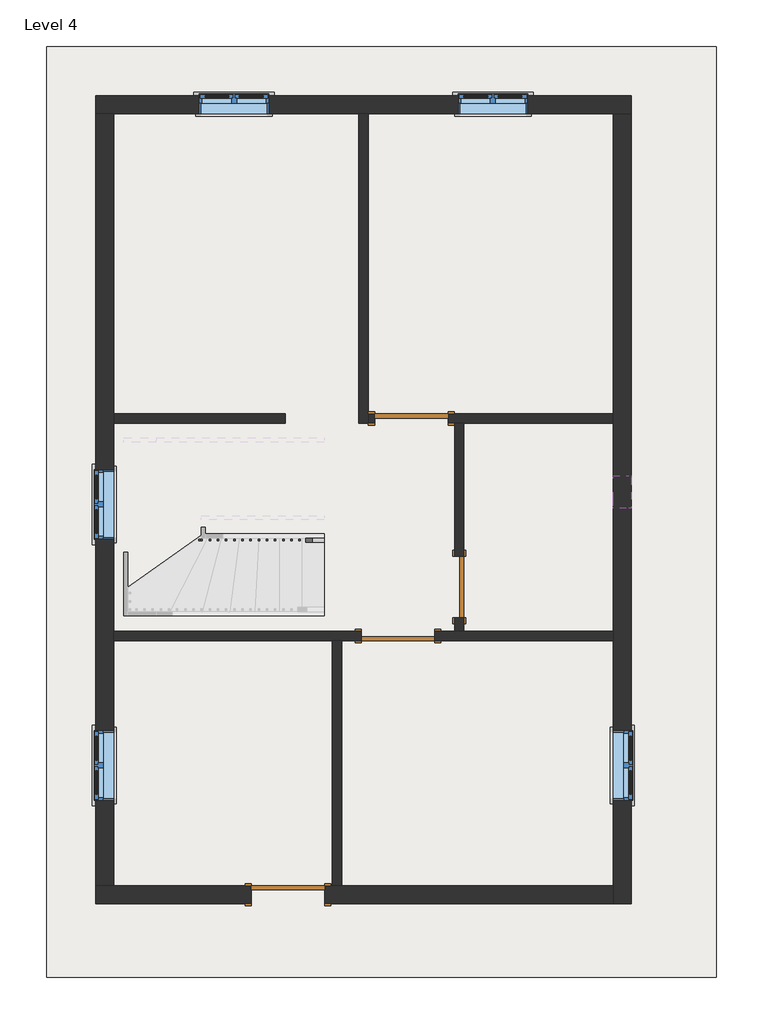
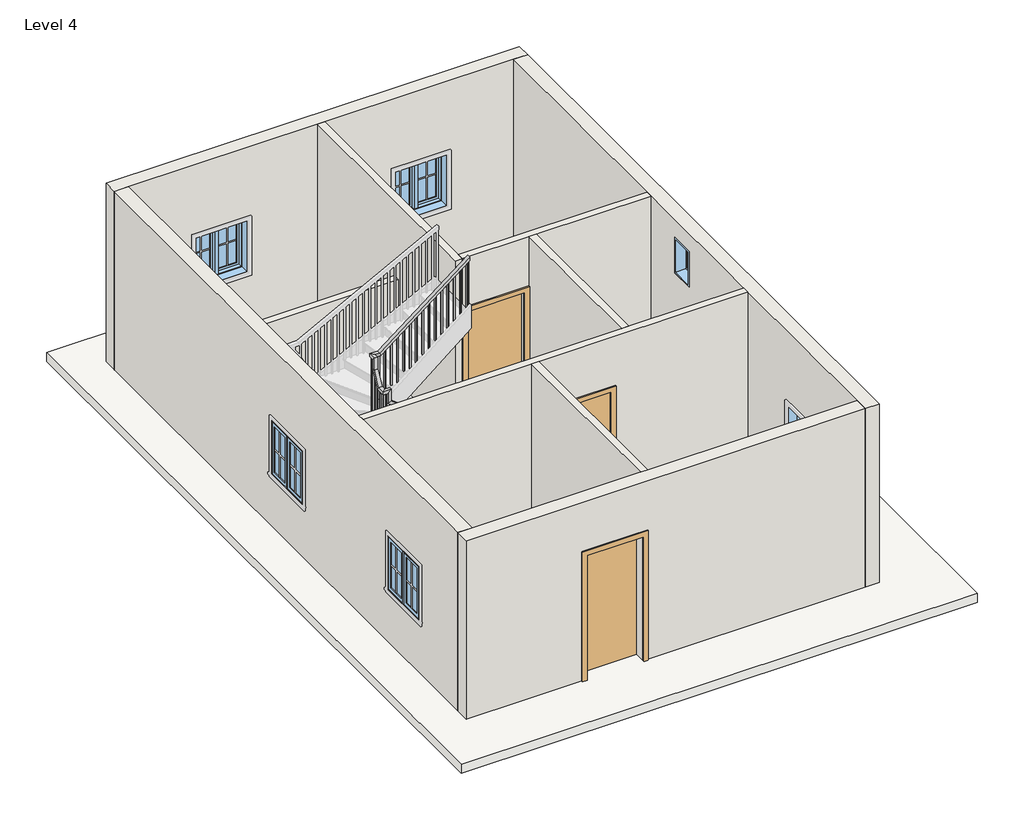
# One storey, part 1 of 2: 10 walls, 6 windows, 4 doors, 1 railing, 1 roof.
"""IFC4 building model written with IfcOpenShell, lengths in millimetres."""

from ifc_helpers import new_model, si_unit, frame, origin, place, context, project, spatial, polyline, outline, extrude, faceted_brep, transform, mapped, element, save
from components import door_d8f5dbb5, door_305aa2a5, door_e5f9f3c4, door_a90ba1ad, window_aa618e30, window_339605e1

model = new_model("IFC4")

# Units and contexts
model_context = context("Model", 3, world=origin())
ifc_project = project(units=[si_unit("LENGTHUNIT", "METRE", prefix="MILLI")], contexts=[model_context])

# Site, building, storey
site = spatial("IfcSite", under=ifc_project)
building = spatial("IfcBuilding", under=site)
storey = spatial("IfcBuildingStorey", under=building, Name="Level 4", Elevation=6400.8)

# Doors
placement = place(None, origin())
door_shape = door_d8f5dbb5(model_context)
element("IfcDoor", 1, ObjectType="Single-Flush : 30\" x 80\"", at=placement, inside=storey, context=model_context, shape_type="MappedRepresentation", body=[
    mapped(door_shape, transform((-82.2715692, -955.3070853, 6400.8), x_axis=(0.0, -1.0, 0.0), y_axis=(1.0, 0.0, 0.0), z_axis=(0.0, 0.0, 1.0))),
])
door_2_shape = door_305aa2a5(model_context)
element("IfcDoor", 2, ObjectType="Single-Flush : 36\" x 84\"", at=placement, inside=storey, context=model_context, shape_type="MappedRepresentation", body=[
    mapped(door_2_shape, transform((-677.5332429, 1140.1929147, 6400.8), x_axis=(-1.0, 0.0, 0.0), y_axis=(0.0, -1.0, 0.0), z_axis=(0.0, 0.0, 1.0))),
])
door_3_shape = door_e5f9f3c4(model_context)
element("IfcDoor", 3, ObjectType="Single-Flush : 36\" x 84\"", at=placement, inside=storey, context=model_context, shape_type="MappedRepresentation", body=[
    mapped(door_3_shape, transform((-842.6332429, -1564.9070853, 6400.8), x_axis=(-1.0, 0.0, 0.0), y_axis=(0.0, -1.0, 0.0), z_axis=(0.0, 0.0, 1.0))),
])
door_4_shape = door_a90ba1ad(model_context)
element("IfcDoor", 4, ObjectType="Single-Flush : 36\" x 84\"", at=placement, inside=storey, context=model_context, shape_type="MappedRepresentation", body=[
    mapped(door_4_shape, transform((-2212.5949167, -4784.3570853, 6400.8), x_axis=(-1.0, 0.0, 0.0), y_axis=(0.0, -1.0, 0.0), z_axis=(0.0, 0.0, 1.0))),
])

# Railing
element("IfcRailing", 5, ObjectType="Handrail - Rectangular", at=placement, inside=storey, context=model_context, shape_type="SolidModel", body=[
    faceted_brep([(-1761.7449167, -396.5070853, 7484.5333333), (-1761.7449167, -396.5070853, 7420.2000346), (-1761.7449167, -345.7070853, 7420.2000346), (-1761.7449167, -345.7070853, 7484.5333333), (-3213.2766085, -396.5070853, 8612.4191036), (-3264.0766085, -396.5070853, 8587.5590024), (-3264.0766085, -345.7070853, 8587.5590024), (-3213.2766085, -345.7070853, 8612.4191036), (-3213.2766085, -396.5070853, 8815.4281882), (-3264.0766085, -396.5070853, 8764.6281882), (-3264.0766085, -345.7070853, 8764.6281882), (-3213.2766085, -345.7070853, 8815.4281882), (-3340.2766085, -396.5070853, 8815.4281882), (-3340.2766085, -396.5070853, 8764.6281882), (-3289.4766085, -345.7070853, 8764.6281882), (-3289.4766085, -345.7070853, 8815.4281882), (-3340.2766085, -269.5070853, 8815.4281882), (-3340.2766085, -240.3857515, 8764.6281882), (-3289.4766085, -240.3857515, 8764.6281882), (-3289.4766085, -269.5070853, 8815.4281882), (-3340.2766085, -142.5070853, 9032.3051451), (-3340.2766085, -91.7070853, 9018.5256424), (-3289.4766085, -91.7070853, 9018.5256424), (-3289.4766085, -142.5070853, 9032.3051451), (-3340.2766085, -142.5070853, 9235.3142297), (-3340.2766085, -91.7070853, 9184.5142297), (-3289.4766085, -91.7070853, 9184.5142297), (-3289.4766085, -142.5070853, 9235.3142297), (-3340.2766085, -15.5070853, 9235.3142297), (-3340.2766085, -15.5070853, 9184.5142297), (-3289.4766085, -66.3070853, 9184.5142297), (-3289.4766085, -66.3070853, 9235.3142297), (-3213.2766085, -15.5070853, 9235.3142297), (-3195.8599406, -15.5070853, 9184.5142297), (-3195.8599406, -66.3070853, 9184.5142297), (-3213.2766085, -66.3070853, 9235.3142297), (-1761.7449167, -15.5070853, 10363.2), (-1761.7449167, -66.3070853, 10363.2), (-1761.7449167, -66.3070853, 10298.8667013), (-1761.7449167, -15.5070853, 10298.8667013)], [[[0, 1, 2, 3]], [[1, 0, 4, 5]], [[2, 1, 5, 6]], [[3, 2, 6, 7]], [[0, 3, 7, 4]], [[5, 4, 8, 9]], [[6, 5, 9, 10]], [[7, 6, 10, 11]], [[4, 7, 11, 8]], [[9, 8, 12, 13]], [[10, 9, 13, 14]], [[11, 10, 14, 15]], [[8, 11, 15, 12]], [[13, 12, 16, 17]], [[14, 13, 17, 18]], [[15, 14, 18, 19]], [[12, 15, 19, 16]], [[17, 16, 20, 21]], [[18, 17, 21, 22]], [[19, 18, 22, 23]], [[16, 19, 23, 20]], [[21, 20, 24, 25]], [[22, 21, 25, 26]], [[23, 22, 26, 27]], [[20, 23, 27, 24]], [[25, 24, 28, 29]], [[26, 25, 29, 30]], [[27, 26, 30, 31]], [[24, 27, 31, 28]], [[29, 28, 32, 33]], [[30, 29, 33, 34]], [[31, 30, 34, 35]], [[28, 31, 35, 32]], [[36, 37, 38, 39]], [[33, 32, 36, 39]], [[34, 33, 39, 38]], [[35, 34, 38, 37]], [[32, 35, 37, 36]]]),
    extrude(outline(polyline([(10283.6316852, -1781.3516085), (10268.8292361, -1800.4016085), (9279.4666667, -1800.4016085), (9279.4666667, -1781.3516085), (10283.6316852, -1781.3516085)])), frame((0.0, -50.4320853, 0.0), z_axis=(0.0, 1.0, 0.0), x_axis=(0.0, 0.0, 1.0)), (0.0, 0.0, 1.0), 19.05),
    extrude(outline(polyline([(10204.6852902, -1882.9516085), (10189.8828411, -1902.0016085), (9279.4666667, -1902.0016085), (9279.4666667, -1882.9516085), (10204.6852902, -1882.9516085)])), frame((0.0, -50.4320853, 0.0), z_axis=(0.0, 1.0, 0.0), x_axis=(0.0, 0.0, 1.0)), (0.0, 0.0, 1.0), 19.05),
    extrude(outline(polyline([(10125.7388952, -1984.5516085), (10110.9364462, -2003.6016085), (9279.4666667, -2003.6016085), (9279.4666667, -1984.5516085), (10125.7388952, -1984.5516085)])), frame((0.0, -50.4320853, 0.0), z_axis=(0.0, 1.0, 0.0), x_axis=(0.0, 0.0, 1.0)), (0.0, 0.0, 1.0), 19.05),
    extrude(outline(polyline([(10046.7925003, -2086.1516085), (10031.9900512, -2105.2016085), (9110.1333333, -2105.2016085), (9110.1333333, -2086.1516085), (10046.7925003, -2086.1516085)])), frame((0.0, -50.4320853, 0.0), z_axis=(0.0, 1.0, 0.0), x_axis=(0.0, 0.0, 1.0)), (0.0, 0.0, 1.0), 19.05),
    extrude(outline(polyline([(9967.8461053, -2187.7516085), (9953.0436562, -2206.8016085), (9110.1333333, -2206.8016085), (9110.1333333, -2187.7516085), (9967.8461053, -2187.7516085)])), frame((0.0, -50.4320853, 0.0), z_axis=(0.0, 1.0, 0.0), x_axis=(0.0, 0.0, 1.0)), (0.0, 0.0, 1.0), 19.05),
    extrude(outline(polyline([(9888.8997103, -2289.3516085), (9874.0972613, -2308.4016085), (9110.1333333, -2308.4016085), (9110.1333333, -2289.3516085), (9888.8997103, -2289.3516085)])), frame((0.0, -50.4320853, 0.0), z_axis=(0.0, 1.0, 0.0), x_axis=(0.0, 0.0, 1.0)), (0.0, 0.0, 1.0), 19.05),
    extrude(outline(polyline([(9809.9533154, -2390.9516085), (9795.1508663, -2410.0016085), (8940.8, -2410.0016085), (8940.8, -2390.9516085), (9809.9533154, -2390.9516085)])), frame((0.0, -50.4320853, 0.0), z_axis=(0.0, 1.0, 0.0), x_axis=(0.0, 0.0, 1.0)), (0.0, 0.0, 1.0), 19.05),
    extrude(outline(polyline([(9731.0069204, -2492.5516085), (9716.2044713, -2511.6016085), (8940.8, -2511.6016085), (8940.8, -2492.5516085), (9731.0069204, -2492.5516085)])), frame((0.0, -50.4320853, 0.0), z_axis=(0.0, 1.0, 0.0), x_axis=(0.0, 0.0, 1.0)), (0.0, 0.0, 1.0), 19.05),
    extrude(outline(polyline([(9652.0605254, -2594.1516085), (9637.2580764, -2613.2016085), (8771.4666667, -2613.2016085), (8771.4666667, -2594.1516085), (9652.0605254, -2594.1516085)])), frame((0.0, -50.4320853, 0.0), z_axis=(0.0, 1.0, 0.0), x_axis=(0.0, 0.0, 1.0)), (0.0, 0.0, 1.0), 19.05),
    extrude(outline(polyline([(9573.1141304, -2695.7516085), (9558.3116814, -2714.8016085), (8771.4666667, -2714.8016085), (8771.4666667, -2695.7516085), (9573.1141304, -2695.7516085)])), frame((0.0, -50.4320853, 0.0), z_axis=(0.0, 1.0, 0.0), x_axis=(0.0, 0.0, 1.0)), (0.0, 0.0, 1.0), 19.05),
    extrude(outline(polyline([(9494.1677355, -2797.3516085), (9479.3652864, -2816.4016085), (8771.4666667, -2816.4016085), (8771.4666667, -2797.3516085), (9494.1677355, -2797.3516085)])), frame((0.0, -50.4320853, 0.0), z_axis=(0.0, 1.0, 0.0), x_axis=(0.0, 0.0, 1.0)), (0.0, 0.0, 1.0), 19.05),
    extrude(outline(polyline([(9415.2213405, -2898.9516085), (9400.4188914, -2918.0016085), (8602.1333333, -2918.0016085), (8602.1333333, -2898.9516085), (9415.2213405, -2898.9516085)])), frame((0.0, -50.4320853, 0.0), z_axis=(0.0, 1.0, 0.0), x_axis=(0.0, 0.0, 1.0)), (0.0, 0.0, 1.0), 19.05),
    extrude(outline(polyline([(9336.2749455, -3000.5516085), (9321.4724965, -3019.6016085), (8602.1333333, -3019.6016085), (8602.1333333, -3000.5516085), (9336.2749455, -3000.5516085)])), frame((0.0, -50.4320853, 0.0), z_axis=(0.0, 1.0, 0.0), x_axis=(0.0, 0.0, 1.0)), (0.0, 0.0, 1.0), 19.05),
    extrude(outline(polyline([(9257.3285506, -3102.1516085), (9242.5261015, -3121.2016085), (8432.8, -3121.2016085), (8432.8, -3102.1516085), (9257.3285506, -3102.1516085)])), frame((0.0, -50.4320853, 0.0), z_axis=(0.0, 1.0, 0.0), x_axis=(0.0, 0.0, 1.0)), (0.0, 0.0, 1.0), 19.05),
    extrude(outline(polyline([(9178.3821556, -3203.7516085), (9163.5797065, -3222.8016085), (8432.8, -3222.8016085), (8432.8, -3203.7516085), (9178.3821556, -3203.7516085)])), frame((0.0, -50.4320853, 0.0), z_axis=(0.0, 1.0, 0.0), x_axis=(0.0, 0.0, 1.0)), (0.0, 0.0, 1.0), 19.05),
    extrude(outline(polyline([(-3305.3516085, -75.8320853), (-3324.4016085, -75.8320853), (-3324.4016085, -56.7820853), (-3305.3516085, -56.7820853), (-3305.3516085, -75.8320853)])), frame((0.0, 0.0, 8094.1333333), z_axis=(0.0, 0.0, 1.0), x_axis=(1.0, 0.0, 0.0)), (0.0, 0.0, 1.0), 1090.3808964),
    extrude(outline(polyline([(-177.4320853, 8872.1336964), (-158.3820853, 8904.66524), (-158.3820853, 7924.8), (-177.4320853, 7924.8), (-177.4320853, 8872.1336964)])), frame((-3324.4016085, 0.0, 0.0), z_axis=(1.0, 0.0, 0.0), x_axis=(0.0, 1.0, 0.0)), (0.0, 0.0, 1.0), 19.05),
    extrude(outline(polyline([(-279.0320853, 8698.6321309), (-259.9820853, 8731.1636744), (-259.9820853, 7755.4666667), (-279.0320853, 7755.4666667), (-279.0320853, 8698.6321309)])), frame((-3324.4016085, 0.0, 0.0), z_axis=(1.0, 0.0, 0.0), x_axis=(0.0, 1.0, 0.0)), (0.0, 0.0, 1.0), 19.05),
    extrude(outline(polyline([(-3276.2199167, -361.5820853), (-3276.2199167, -380.6320853), (-3295.2699167, -380.6320853), (-3295.2699167, -361.5820853), (-3276.2199167, -361.5820853)])), frame((0.0, 0.0, 7586.1333333), z_axis=(0.0, 0.0, 1.0), x_axis=(1.0, 0.0, 0.0)), (0.0, 0.0, 1.0), 1178.4948549),
    extrude(outline(polyline([(8518.0483397, -3174.6199167), (8532.8507888, -3193.6699167), (7416.8, -3193.6699167), (7416.8, -3174.6199167), (8518.0483397, -3174.6199167)])), frame((0.0, -380.6320853, 0.0), z_axis=(0.0, 1.0, 0.0), x_axis=(0.0, 0.0, 1.0)), (0.0, 0.0, 1.0), 19.05),
    extrude(outline(polyline([(8439.1019447, -3073.0199167), (8453.9043938, -3092.0699167), (7416.8, -3092.0699167), (7416.8, -3073.0199167), (8439.1019447, -3073.0199167)])), frame((0.0, -380.6320853, 0.0), z_axis=(0.0, 1.0, 0.0), x_axis=(0.0, 0.0, 1.0)), (0.0, 0.0, 1.0), 19.05),
    extrude(outline(polyline([(8360.1555498, -2971.4199167), (8374.9579988, -2990.4699167), (7247.4666667, -2990.4699167), (7247.4666667, -2971.4199167), (8360.1555498, -2971.4199167)])), frame((0.0, -380.6320853, 0.0), z_axis=(0.0, 1.0, 0.0), x_axis=(0.0, 0.0, 1.0)), (0.0, 0.0, 1.0), 19.05),
    extrude(outline(polyline([(8281.2091548, -2869.8199167), (8296.0116039, -2888.8699167), (7247.4666667, -2888.8699167), (7247.4666667, -2869.8199167), (8281.2091548, -2869.8199167)])), frame((0.0, -380.6320853, 0.0), z_axis=(0.0, 1.0, 0.0), x_axis=(0.0, 0.0, 1.0)), (0.0, 0.0, 1.0), 19.05),
    extrude(outline(polyline([(8202.2627598, -2768.2199167), (8217.0652089, -2787.2699167), (7078.1333333, -2787.2699167), (7078.1333333, -2768.2199167), (8202.2627598, -2768.2199167)])), frame((0.0, -380.6320853, 0.0), z_axis=(0.0, 1.0, 0.0), x_axis=(0.0, 0.0, 1.0)), (0.0, 0.0, 1.0), 19.05),
    extrude(outline(polyline([(8123.3163649, -2666.6199167), (8138.1188139, -2685.6699167), (7078.1333333, -2685.6699167), (7078.1333333, -2666.6199167), (8123.3163649, -2666.6199167)])), frame((0.0, -380.6320853, 0.0), z_axis=(0.0, 1.0, 0.0), x_axis=(0.0, 0.0, 1.0)), (0.0, 0.0, 1.0), 19.05),
    extrude(outline(polyline([(8044.3699699, -2565.0199167), (8059.1724189, -2584.0699167), (6908.8, -2584.0699167), (6908.8, -2565.0199167), (8044.3699699, -2565.0199167)])), frame((0.0, -380.6320853, 0.0), z_axis=(0.0, 1.0, 0.0), x_axis=(0.0, 0.0, 1.0)), (0.0, 0.0, 1.0), 19.05),
    extrude(outline(polyline([(7965.4235749, -2463.4199167), (7980.226024, -2482.4699167), (6908.8, -2482.4699167), (6908.8, -2463.4199167), (7965.4235749, -2463.4199167)])), frame((0.0, -380.6320853, 0.0), z_axis=(0.0, 1.0, 0.0), x_axis=(0.0, 0.0, 1.0)), (0.0, 0.0, 1.0), 19.05),
    extrude(outline(polyline([(7886.4771799, -2361.8199167), (7901.279629, -2380.8699167), (6908.8, -2380.8699167), (6908.8, -2361.8199167), (7886.4771799, -2361.8199167)])), frame((0.0, -380.6320853, 0.0), z_axis=(0.0, 1.0, 0.0), x_axis=(0.0, 0.0, 1.0)), (0.0, 0.0, 1.0), 19.05),
    extrude(outline(polyline([(7807.530785, -2260.2199167), (7822.333234, -2279.2699167), (6739.4666667, -2279.2699167), (6739.4666667, -2260.2199167), (7807.530785, -2260.2199167)])), frame((0.0, -380.6320853, 0.0), z_axis=(0.0, 1.0, 0.0), x_axis=(0.0, 0.0, 1.0)), (0.0, 0.0, 1.0), 19.05),
    extrude(outline(polyline([(7728.58439, -2158.6199167), (7743.3868391, -2177.6699167), (6739.4666667, -2177.6699167), (6739.4666667, -2158.6199167), (7728.58439, -2158.6199167)])), frame((0.0, -380.6320853, 0.0), z_axis=(0.0, 1.0, 0.0), x_axis=(0.0, 0.0, 1.0)), (0.0, 0.0, 1.0), 19.05),
    extrude(outline(polyline([(7649.637995, -2057.0199167), (7664.4404441, -2076.0699167), (6739.4666667, -2076.0699167), (6739.4666667, -2057.0199167), (7649.637995, -2057.0199167)])), frame((0.0, -380.6320853, 0.0), z_axis=(0.0, 1.0, 0.0), x_axis=(0.0, 0.0, 1.0)), (0.0, 0.0, 1.0), 19.05),
    extrude(outline(polyline([(7570.6916001, -1955.4199167), (7585.4940491, -1974.4699167), (6570.1333333, -1974.4699167), (6570.1333333, -1955.4199167), (7570.6916001, -1955.4199167)])), frame((0.0, -380.6320853, 0.0), z_axis=(0.0, 1.0, 0.0), x_axis=(0.0, 0.0, 1.0)), (0.0, 0.0, 1.0), 19.05),
    extrude(outline(polyline([(7491.7452051, -1853.8199167), (7506.5476541, -1872.8699167), (6570.1333333, -1872.8699167), (6570.1333333, -1853.8199167), (7491.7452051, -1853.8199167)])), frame((0.0, -380.6320853, 0.0), z_axis=(0.0, 1.0, 0.0), x_axis=(0.0, 0.0, 1.0)), (0.0, 0.0, 1.0), 19.05),
    extrude(outline(polyline([(-3305.3516085, -50.4320853), (-3324.4016085, -50.4320853), (-3324.4016085, -31.3820853), (-3305.3516085, -31.3820853), (-3305.3516085, -50.4320853)])), frame((0.0, 0.0, 8263.4666667), z_axis=(0.0, 0.0, 1.0), x_axis=(1.0, 0.0, 0.0)), (0.0, 0.0, 1.0), 921.0475631),
    extrude(outline(polyline([(-3305.3516085, -361.5820853), (-3305.3516085, -380.6320853), (-3324.4016085, -380.6320853), (-3324.4016085, -361.5820853), (-3305.3516085, -361.5820853)])), frame((0.0, 0.0, 7586.1333333), z_axis=(0.0, 0.0, 1.0), x_axis=(1.0, 0.0, 0.0)), (0.0, 0.0, 1.0), 1178.4948549),
    extrude(outline(polyline([(10298.8667013, -1761.7449167), (10284.0642523, -1780.7949167), (9279.4666667, -1780.7949167), (9279.4666667, -1761.7449167), (10298.8667013, -1761.7449167)])), frame((0.0, -50.4320853, 0.0), z_axis=(0.0, 1.0, 0.0), x_axis=(0.0, 0.0, 1.0)), (0.0, 0.0, 1.0), 19.05),
    extrude(outline(polyline([(7420.2000346, -1761.7449167), (7435.0024837, -1780.7949167), (6570.1333333, -1780.7949167), (6570.1333333, -1761.7449167), (7420.2000346, -1761.7449167)])), frame((0.0, -380.6320853, 0.0), z_axis=(0.0, 1.0, 0.0), x_axis=(0.0, 0.0, 1.0)), (0.0, 0.0, 1.0), 19.05),
])

# Roof
element("IfcRoof", 6, ObjectType="Generic - 12\"", at=placement, inside=storey, context=model_context, shape_type="SweptSolid", body=[
    extrude(outline(polyline([(-5216.1449167, 5769.3429147), (3115.0550833, 5769.3429147), (3115.0550833, -5813.0570853), (-5216.1449167, -5813.0570853), (-5216.1449167, 5769.3429147)])), frame((0.0, 0.0, 6248.4), z_axis=(0.0, 0.0, 1.0), x_axis=(1.0, 0.0, 0.0)), (0.0, 0.0, 1.0), 152.4),
])

# Walls
element("IfcWall", 7, ObjectType="WALL4.5\"", at=placement, inside=storey, context=model_context, shape_type="Brep", body=[
    faceted_brep([(-1329.9449167, 4931.1429147, 6400.8), (-1329.9449167, 1083.0429147, 6400.8), (-1329.9449167, 1083.0429147, 9448.8), (-1329.9449167, 4931.1429147, 9448.8), (-1215.6449167, 4931.1429147, 6400.8), (-1215.6449167, 4931.1429147, 9448.8), (-1215.6449167, 1197.3429147, 9448.8), (-1215.6449167, 1083.0429147, 9448.8), (-1215.6449167, 1083.0429147, 6400.8), (-1215.6449167, 1197.3429147, 6400.8)], [[[0, 1, 2, 3]], [[4, 5, 6, 7, 8, 9]], [[1, 0, 4, 9, 8]], [[0, 3, 5, 4]], [[2, 1, 8, 7]], [[3, 2, 7, 6, 5]]]),
])
element("IfcWall", 8, ObjectType="WALL4.5\"", at=placement, inside=storey, context=model_context, shape_type="Brep", body=[
    faceted_brep([(-1215.6449167, 1083.0429147, 6400.8), (-1134.7332429, 1083.0429147, 6400.8), (-1134.7332429, 1083.0429147, 8534.4), (-220.3332429, 1083.0429147, 8534.4), (-220.3332429, 1083.0429147, 6400.8), (-139.4215692, 1083.0429147, 6400.8), (-25.1215692, 1083.0429147, 6400.8), (1832.3550833, 1083.0429147, 6400.8), (1832.3550833, 1083.0429147, 9448.8), (-25.1215692, 1083.0429147, 9448.8), (-139.4215692, 1083.0429147, 9448.8), (-1215.6449167, 1083.0429147, 9448.8), (-1134.7332429, 1197.3429147, 8534.4), (-1134.7332429, 1197.3429147, 6400.8), (-1215.6449167, 1197.3429147, 6400.8), (-1215.6449167, 1197.3429147, 9448.8), (1832.3550833, 1197.3429147, 9448.8), (1832.3550833, 1197.3429147, 6400.8), (-220.3332429, 1197.3429147, 6400.8), (-220.3332429, 1197.3429147, 8534.4)], [[[0, 1, 2, 3, 4, 5, 6, 7, 8, 9, 10, 11]], [[12, 13, 14, 15, 16, 17, 18, 19]], [[18, 17, 7, 6, 5, 4]], [[14, 13, 1, 0]], [[0, 11, 15, 14]], [[8, 7, 17, 16]], [[2, 1, 13, 12]], [[3, 2, 12, 19]], [[4, 3, 19, 18]], [[11, 10, 9, 8, 16, 15]]]),
])
element("IfcWall", 9, ObjectType="WALL4.5\"", at=placement, inside=storey, context=model_context, shape_type="SweptSolid", body=[
    extrude(outline(polyline([(-2244.3449167, 1083.0429147), (-4377.9449167, 1083.0429147), (-4377.9449167, 1197.3429147), (-2244.3449167, 1197.3429147), (-2244.3449167, 1083.0429147)])), frame((0.0, 0.0, 6400.8), z_axis=(0.0, 0.0, 1.0), x_axis=(1.0, 0.0, 0.0)), (0.0, 0.0, 1.0), 3048.0),
])
element("IfcWall", 10, ObjectType="WALL4.5\"", at=placement, inside=storey, context=model_context, shape_type="SweptSolid", body=[
    extrude(outline(polyline([(-1336.3070853, 8432.8), (-1336.3070853, 6400.8), (-1507.7570853, 6400.8), (-1507.7570853, 9448.8), (1083.0429147, 9448.8), (1083.0429147, 6400.8), (-574.3070853, 6400.8), (-574.3070853, 8432.8), (-1336.3070853, 8432.8)])), frame((-139.4215692, 0.0, 0.0), z_axis=(1.0, 0.0, 0.0), x_axis=(0.0, 1.0, 0.0)), (0.0, 0.0, 1.0), 114.3),
])
element("IfcWall", 11, ObjectType="WALL4.5\"", at=placement, inside=storey, context=model_context, shape_type="Brep", body=[
    faceted_brep([(-4377.9449167, -1622.0570853, 6400.8), (-1660.1449167, -1622.0570853, 6400.8), (-1545.8449167, -1622.0570853, 6400.8), (-1299.8332429, -1622.0570853, 6400.8), (-1299.8332429, -1622.0570853, 8534.4), (-385.4332429, -1622.0570853, 8534.4), (-385.4332429, -1622.0570853, 6400.8), (1832.3550833, -1622.0570853, 6400.8), (1832.3550833, -1622.0570853, 9448.8), (-1545.8449167, -1622.0570853, 9448.8), (-1660.1449167, -1622.0570853, 9448.8), (-4377.9449167, -1622.0570853, 9448.8), (-1299.8332429, -1507.7570853, 8534.4), (-1299.8332429, -1507.7570853, 6400.8), (-4377.9449167, -1507.7570853, 6400.8), (-4377.9449167, -1507.7570853, 9448.8), (-139.4215692, -1507.7570853, 9448.8), (-25.1215692, -1507.7570853, 9448.8), (1832.3550833, -1507.7570853, 9448.8), (1832.3550833, -1507.7570853, 6400.8), (-25.1215692, -1507.7570853, 6400.8), (-139.4215692, -1507.7570853, 6400.8), (-385.4332429, -1507.7570853, 6400.8), (-385.4332429, -1507.7570853, 8534.4)], [[[0, 1, 2, 3, 4, 5, 6, 7, 8, 9, 10, 11]], [[12, 13, 14, 15, 16, 17, 18, 19, 20, 21, 22, 23]], [[14, 13, 3, 2, 1, 0]], [[22, 21, 20, 19, 7, 6]], [[8, 7, 19, 18]], [[0, 11, 15, 14]], [[4, 3, 13, 12]], [[5, 4, 12, 23]], [[6, 5, 23, 22]], [[11, 10, 9, 8, 18, 17, 16, 15]]]),
])
element("IfcWall", 12, ObjectType="WALL4.5\"", at=placement, inside=storey, context=model_context, shape_type="SweptSolid", body=[
    extrude(outline(polyline([(-1660.1449167, -4670.0570853), (-1660.1449167, -1622.0570853), (-1545.8449167, -1622.0570853), (-1545.8449167, -4670.0570853), (-1660.1449167, -4670.0570853)])), frame((0.0, 0.0, 6400.8), z_axis=(0.0, 0.0, 1.0), x_axis=(1.0, 0.0, 0.0)), (0.0, 0.0, 1.0), 3048.0),
])
element("IfcWall", 13, ObjectType="WALL9\"", at=placement, inside=storey, context=model_context, shape_type="Brep", body=[
    faceted_brep([(-4606.5449167, 4931.1429147, 6400.8), (-4377.9449167, 4931.1429147, 6400.8), (-1329.9449167, 4931.1429147, 6400.8), (-1215.6449167, 4931.1429147, 6400.8), (1832.3550833, 4931.1429147, 6400.8), (2060.9550833, 4931.1429147, 6400.8), (2060.9550833, 4931.1429147, 9448.8), (1832.3550833, 4931.1429147, 9448.8), (-1215.6449167, 4931.1429147, 9448.8), (-1329.9449167, 4931.1429147, 9448.8), (-4377.9449167, 4931.1429147, 9448.8), (-4606.5449167, 4931.1429147, 9448.8), (-2450.7199167, 4931.1429147, 8229.6), (-2450.7199167, 4931.1429147, 7315.2), (-3314.3199167, 4931.1429147, 7315.2), (-3314.3199167, 4931.1429147, 8229.6), (768.7300833, 4931.1429147, 8229.6), (768.7300833, 4931.1429147, 7315.2), (-94.8699167, 4931.1429147, 7315.2), (-94.8699167, 4931.1429147, 8229.6), (-4606.5449167, 5159.7429147, 6400.8), (-4606.5449167, 5159.7429147, 9448.8), (2060.9550833, 5159.7429147, 9448.8), (2060.9550833, 5159.7429147, 6400.8), (-2450.7199167, 5159.7429147, 8229.6), (-3314.3199167, 5159.7429147, 8229.6), (-3314.3199167, 5159.7429147, 7315.2), (-2450.7199167, 5159.7429147, 7315.2), (768.7300833, 5159.7429147, 8229.6), (-94.8699167, 5159.7429147, 8229.6), (-94.8699167, 5159.7429147, 7315.2), (768.7300833, 5159.7429147, 7315.2)], [[[0, 1, 2, 3, 4, 5, 6, 7, 8, 9, 10, 11], [12, 13, 14, 15], [16, 17, 18, 19]], [[20, 21, 22, 23], [24, 25, 26, 27], [28, 29, 30, 31]], [[5, 4, 3, 2, 1, 0, 20, 23]], [[6, 5, 23, 22]], [[0, 11, 21, 20]], [[13, 12, 24, 27]], [[14, 13, 27, 26]], [[15, 14, 26, 25]], [[12, 15, 25, 24]], [[17, 16, 28, 31]], [[18, 17, 31, 30]], [[19, 18, 30, 29]], [[16, 19, 29, 28]], [[11, 10, 9, 8, 7, 6, 22, 21]]]),
])
element("IfcWall", 14, ObjectType="WALL9\"", at=placement, inside=storey, context=model_context, shape_type="Brep", body=[
    faceted_brep([(1832.3550833, 4931.1429147, 6400.8), (1832.3550833, 1197.3429147, 6400.8), (1832.3550833, 1083.0429147, 6400.8), (1832.3550833, -1507.7570853, 6400.8), (1832.3550833, -1622.0570853, 6400.8), (1832.3550833, -4670.0570853, 6400.8), (1832.3550833, -4898.6570853, 6400.8), (1832.3550833, -4898.6570853, 9448.8), (1832.3550833, -4670.0570853, 9448.8), (1832.3550833, -1622.0570853, 9448.8), (1832.3550833, -1507.7570853, 9448.8), (1832.3550833, 1083.0429147, 9448.8), (1832.3550833, 1197.3429147, 9448.8), (1832.3550833, 4931.1429147, 9448.8), (1832.3550833, 22.5929147, 9144.0), (1832.3550833, 22.5929147, 8534.4), (1832.3550833, 428.9929147, 8534.4), (1832.3550833, 428.9929147, 9144.0), (1832.3550833, -3606.4320853, 8229.6), (1832.3550833, -3606.4320853, 7315.2), (1832.3550833, -2742.8320853, 7315.2), (1832.3550833, -2742.8320853, 8229.6), (2060.9550833, 4931.1429147, 6400.8), (2060.9550833, 4931.1429147, 9448.8), (2060.9550833, -4898.6570853, 9448.8), (2060.9550833, -4898.6570853, 6400.8), (2060.9550833, 22.5929147, 9144.0), (2060.9550833, 428.9929147, 9144.0), (2060.9550833, 428.9929147, 8534.4), (2060.9550833, 22.5929147, 8534.4), (2060.9550833, -3606.4320853, 8229.6), (2060.9550833, -2742.8320853, 8229.6), (2060.9550833, -2742.8320853, 7315.2), (2060.9550833, -3606.4320853, 7315.2)], [[[0, 1, 2, 3, 4, 5, 6, 7, 8, 9, 10, 11, 12, 13], [14, 15, 16, 17], [18, 19, 20, 21]], [[22, 23, 24, 25], [26, 27, 28, 29], [30, 31, 32, 33]], [[6, 5, 4, 3, 2, 1, 0, 22, 25]], [[0, 13, 23, 22]], [[7, 6, 25, 24]], [[15, 14, 26, 29]], [[16, 15, 29, 28]], [[17, 16, 28, 27]], [[14, 17, 27, 26]], [[19, 18, 30, 33]], [[20, 19, 33, 32]], [[21, 20, 32, 31]], [[18, 21, 31, 30]], [[13, 12, 11, 10, 9, 8, 7, 24, 23]]]),
])
element("IfcWall", 15, ObjectType="WALL9\"", at=placement, inside=storey, context=model_context, shape_type="Brep", body=[
    faceted_brep([(-2669.7949167, -4670.0570853, 8534.4), (-2669.7949167, -4670.0570853, 6400.8), (-4377.9449167, -4670.0570853, 6400.8), (-4606.5449167, -4670.0570853, 6400.8), (-4606.5449167, -4670.0570853, 9448.8), (-4377.9449167, -4670.0570853, 9448.8), (-1660.1449167, -4670.0570853, 9448.8), (-1545.8449167, -4670.0570853, 9448.8), (1832.3550833, -4670.0570853, 9448.8), (1832.3550833, -4670.0570853, 6400.8), (-1545.8449167, -4670.0570853, 6400.8), (-1660.1449167, -4670.0570853, 6400.8), (-1755.3949167, -4670.0570853, 6400.8), (-1755.3949167, -4670.0570853, 8534.4), (-4606.5449167, -4898.6570853, 6400.8), (-2669.7949167, -4898.6570853, 6400.8), (-2669.7949167, -4898.6570853, 8534.4), (-1755.3949167, -4898.6570853, 8534.4), (-1755.3949167, -4898.6570853, 6400.8), (1832.3550833, -4898.6570853, 6400.8), (1832.3550833, -4898.6570853, 9448.8), (-4606.5449167, -4898.6570853, 9448.8)], [[[0, 1, 2, 3, 4, 5, 6, 7, 8, 9, 10, 11, 12, 13]], [[14, 15, 16, 17, 18, 19, 20, 21]], [[3, 2, 1, 15, 14]], [[12, 11, 10, 9, 19, 18]], [[9, 8, 20, 19]], [[4, 3, 14, 21]], [[16, 15, 1, 0]], [[17, 16, 0, 13]], [[18, 17, 13, 12]], [[8, 7, 6, 5, 4, 21, 20]]]),
])
element("IfcWall", 16, ObjectType="WALL9\"", at=placement, inside=storey, context=model_context, shape_type="Brep", body=[
    faceted_brep([(-4377.9449167, -4670.0570853, 6400.8), (-4377.9449167, -1622.0570853, 6400.8), (-4377.9449167, -1507.7570853, 6400.8), (-4377.9449167, 1083.0429147, 6400.8), (-4377.9449167, 1197.3429147, 6400.8), (-4377.9449167, 4931.1429147, 6400.8), (-4377.9449167, 4931.1429147, 9448.8), (-4377.9449167, 1197.3429147, 9448.8), (-4377.9449167, 1083.0429147, 9448.8), (-4377.9449167, -1507.7570853, 9448.8), (-4377.9449167, -1622.0570853, 9448.8), (-4377.9449167, -4670.0570853, 9448.8), (-4377.9449167, -2742.8320853, 8229.6), (-4377.9449167, -2742.8320853, 7315.2), (-4377.9449167, -3606.4320853, 7315.2), (-4377.9449167, -3606.4320853, 8229.6), (-4377.9449167, 505.1929147, 8229.6), (-4377.9449167, 505.1929147, 7315.2), (-4377.9449167, -358.4070853, 7315.2), (-4377.9449167, -358.4070853, 8229.6), (-4606.5449167, -4670.0570853, 6400.8), (-4606.5449167, -4670.0570853, 9448.8), (-4606.5449167, 4931.1429147, 9448.8), (-4606.5449167, 4931.1429147, 6400.8), (-4606.5449167, -2742.8320853, 8229.6), (-4606.5449167, -3606.4320853, 8229.6), (-4606.5449167, -3606.4320853, 7315.2), (-4606.5449167, -2742.8320853, 7315.2), (-4606.5449167, 505.1929147, 8229.6), (-4606.5449167, -358.4070853, 8229.6), (-4606.5449167, -358.4070853, 7315.2), (-4606.5449167, 505.1929147, 7315.2)], [[[0, 1, 2, 3, 4, 5, 6, 7, 8, 9, 10, 11], [12, 13, 14, 15], [16, 17, 18, 19]], [[20, 21, 22, 23], [24, 25, 26, 27], [28, 29, 30, 31]], [[5, 4, 3, 2, 1, 0, 20, 23]], [[0, 11, 21, 20]], [[6, 5, 23, 22]], [[13, 12, 24, 27]], [[14, 13, 27, 26]], [[15, 14, 26, 25]], [[12, 15, 25, 24]], [[17, 16, 28, 31]], [[18, 17, 31, 30]], [[19, 18, 30, 29]], [[16, 19, 29, 28]], [[11, 10, 9, 8, 7, 6, 22, 21]]]),
])

# Windows
window_shape = window_aa618e30(model_context)
element("IfcWindow", 17, ObjectType="Fixed : 16\" x 24\"", at=placement, inside=storey, context=model_context, shape_type="MappedRepresentation", body=[
    mapped(window_shape, transform((1946.6550833, 187.6929147, 7620.0), x_axis=(0.0, -1.0, 0.0), y_axis=(1.0, 0.0, 0.0), z_axis=(0.0, 0.0, 1.0))),
])
window_2_shape = window_339605e1(model_context)
element("IfcWindow", 18, ObjectType="Window-Casement-Double : 34\" x 36\"", at=placement, inside=storey, context=model_context, shape_type="MappedRepresentation", body=[
    mapped(window_2_shape, transform((-2882.5199167, 5045.4429147, 6400.8), x_axis=(1.0, 0.0, 0.0), y_axis=(0.0, 1.0, 0.0), z_axis=(0.0, 0.0, 1.0))),
])
element("IfcWindow", 19, ObjectType="Window-Casement-Double : 34\" x 36\"", at=placement, inside=storey, context=model_context, shape_type="MappedRepresentation", body=[
    mapped(window_2_shape, transform((336.9300833, 5045.4429147, 6400.8), x_axis=(1.0, 0.0, 0.0), y_axis=(0.0, 1.0, 0.0), z_axis=(0.0, 0.0, 1.0))),
])
element("IfcWindow", 20, ObjectType="Window-Casement-Double : 34\" x 36\"", at=placement, inside=storey, context=model_context, shape_type="MappedRepresentation", body=[
    mapped(window_2_shape, transform((-4492.2449167, -3174.6320853, 6400.8), x_axis=(0.0, 1.0, 0.0), y_axis=(-1.0, 0.0, 0.0), z_axis=(0.0, 0.0, 1.0))),
])
element("IfcWindow", 21, ObjectType="Window-Casement-Double : 34\" x 36\"", at=placement, inside=storey, context=model_context, shape_type="MappedRepresentation", body=[
    mapped(window_2_shape, transform((1946.6550833, -3174.6320853, 6400.8), x_axis=(0.0, -1.0, 0.0), y_axis=(1.0, 0.0, 0.0), z_axis=(0.0, 0.0, 1.0))),
])
element("IfcWindow", 22, ObjectType="Window-Casement-Double : 34\" x 36\"", at=placement, inside=storey, context=model_context, shape_type="MappedRepresentation", body=[
    mapped(window_2_shape, transform((-4492.2449167, 73.3929147, 6400.8), x_axis=(0.0, 1.0, 0.0), y_axis=(-1.0, 0.0, 0.0), z_axis=(0.0, 0.0, 1.0))),
])

save(model, "model.ifc")

# Revit data of these elements
# Type "Single-Flush : 30\" x 80\""
#   Type Mark = "5"
#   Construction Type Id = "MDOOR"
#   Assembly Code = "C1020"
#   Analytic Construction = "Metal"
#   Thickness = 0' - 2"
#   Heat Transfer Coefficient (U) = 0.651978 BTU/(h·ft²·°F)
#   Height = 6' - 8"
#   Trim Projection Ext = 0' - 1"
#   Trim Projection Int = 0' - 1"
#   Trim Width = 0' - 3"
#   Width = 2' - 6"
#   Define Thermal Properties by = 1
#   Define Thermal Properties by = 1
#   Door Material = Door - Panel
#   Frame Material = Door - Frame
#   Visual Light Transmittance = 0
#   Solar Heat Gain Coefficient = 0
#   Function = (empty or 0)
#   Wall Closure = (empty or 0)
# Type "Single-Flush : 36\" x 84\""
#   Type Mark = "1"
#   Construction Type Id = "MDOOR"
#   Assembly Code = "C1020"
#   Analytic Construction = "Metal"
#   Thickness = 0' - 2"
#   Heat Transfer Coefficient (U) = 0.651978 BTU/(h·ft²·°F)
#   Height = 7' - 0"
#   Trim Projection Ext = 0' - 1"
#   Trim Projection Int = 0' - 1"
#   Trim Width = 0' - 3"
#   Width = 3' - 0"
#   Define Thermal Properties by = 1
#   Define Thermal Properties by = 1
#   Door Material = Door - Panel
#   Frame Material = Door - Frame
#   Visual Light Transmittance = 0
#   Solar Heat Gain Coefficient = 0
#   Function = (empty or 0)
#   Wall Closure = (empty or 0)
# Type "Handrail - Rectangular"
#   Assembly Code = "C2010400"
#   built-in parameter 1008612 = 0.0416667 (stored number, unit not read)
#   built-in parameter 1008611 = 0.0416667 (stored number, unit not read)
#   built-in parameter 1008609 = 0.333333 (stored number, unit not read)
#   built-in parameter 1008604 = 0.166667 (stored number, unit not read)
#   built-in parameter 1008603 = 0.166667 (stored number, unit not read)
#   Railing Height = 3' - 0"
#   built-in parameter 1008630 = 2
#   built-in parameter 1008610 = 2
#   built-in parameter 1008618 = Baluster - Square : 3/4"
# Type "Generic - 12\""
#   Assembly Code = "B1020"
#   Layers, outside or top first: 0' - 6" no material (function 1)
# Type "WALL4.5\""
#   Assembly Code = "B2010"
#   Layers, outside or top first: 0' - 4 1/2" no material (function 1)
# Type "WALL9\""
#   Assembly Code = "B2010"
#   Layers, outside or top first: 0' - 9" no material (function 1)
# Type "Fixed : 16\" x 24\""
#   Type Mark = "4"
#   Construction Type Id = "GSP4R"
#   Assembly Code = "B2020100"
#   Analytic Construction = "1/8 in Pilkington single glazing"
#   Visual Light Transmittance = 0.9
#   Solar Heat Gain Coefficient = 0.78
#   Heat Transfer Coefficient (U) = 0.6496 BTU/(h·ft²·°F)
#   Height = 2' - 0"
#   Default Sill Height = 3' - 0"
#   Width = 1' - 4"
#   Window Inset = 0' - 0 3/4"
#   Define Thermal Properties by = 1
#   Define Thermal Properties by = 1
#   Glass Pane Material = Glass
#   Sash Material = Sash
#   Wall Closure = (empty or 0)
# Type "Window-Casement-Double : 34\" x 36\""
#   Type Mark = "14"
#   Fire Rating = "0.5h"
#   Assembly Code = "B2020100"
#   Analytic Construction = "Double glazing - domestic"
#   Frame Extension [instance default] = 0' - 0 1/4"
#   Window Inset [instance default] = 0' - 0"
#   Wall Thickness [instance default] = 0' - 6"
#   Interior Wall Closure [instance default] = 0' - 2 1/4"
#   Half Width = 1' - 5"
#   Visual Light Transmittance = 0.81
#   Thermal Resistance (R) = 1.8146 (h·ft²·°F)/BTU
#   Solar Heat Gain Coefficient = 0.76
#   Rough Width = 2' - 10 1/2"
#   Rough Height = 3' - 0 1/2"
#   Height = 3' - 0"
#   Heat Transfer Coefficient (U) = 0.5511 BTU/(h·ft²·°F)
#   Exterior Wall Closure [instance default] = 0' - 1 1/4"
#   Extension Jamb [instance default] = 0' - 2 1/4"
#   Default Sill Height = 3' - 0"
#   Width = 2' - 10"
#   Define Thermal Properties by = 0
#   Muntin Visibility = yes
#   Interior Trim Visibility [instance default] = yes
#   Exterior Trim Visibility [instance default] = yes
#   Extension Jamb Visibility [instance default] = yes
#   Interior Trim Material = Wood - Stained
#   Muntin Pattern = Muntin Pattern_2x2 : Muntin Pattern_2x2
#   Interior Trim = Trim-Window-Interior-Flat : Picture Frame
#   Interior Frame Material = Wood - Stained
#   Glass Panel Material = Glass
#   Exterior Trim Material = Clad - White
#   Exterior Trim = Trim-Window-Exterior-Flat : with Sill
#   Exterior Frame Material = Clad - White
#   Wall Closure = (empty or 0)
# Element 1 (IfcDoor, "Single-Flush : 30\" x 80\"")
#   Phase Created = New Construction
#   Materials on its faces: "Door - Frame", "Door - Panel"
# Elements 2, 3, 4 (IfcDoor, "Single-Flush : 36\" x 84\"")
#   Phase Created = New Construction
#   Materials on its faces: "Door - Frame", "Door - Panel"
# Element 5 (IfcRailing, "Handrail - Rectangular")
#   Phase Created = New Construction
# Element 6 (IfcRoof, "Generic - 12\"")
#   built-in parameter 1001705 = 21 (stored number, unit not read)
#   built-in parameter 1001701 = -0.5 (stored number, unit not read)
#   built-in parameter 1001710 = 33615
#   Phase Created = New Construction
#   Materials on its faces: "Default Roof"
# Elements 7, 8, 9, 10, 11, 12 (IfcWall, "WALL4.5\"")
#   Top Offset = 0' - 0"
#   Base Offset = 0' - 0"
#   Unconnected Height = 10' - 0"
#   wall height = 10' - 0"
#   Phase Created = New Construction
#   Base Constraint = Level 4
#   Materials on its faces: "Default Wall"
# Elements 13, 14, 15, 16 (IfcWall, "WALL9\"")
#   Top Offset = 0' - 0"
#   Base Offset = 0' - 0"
#   Unconnected Height = 10' - 0"
#   wall height = 10' - 0"
#   Phase Created = New Construction
#   Base Constraint = Level 4
#   Materials on its faces: "Default Wall", "Brick, Soldier Course"
# Element 17 (IfcWindow, "Fixed : 16\" x 24\"")
#   Mark = "13"
#   Phase Created = New Construction
#   Materials on its faces: "Sash", "Glass"
# Element 18 (IfcWindow, "Window-Casement-Double : 34\" x 36\"")
#   Mark = "14"
#   Window Inset = 0' - 0"
#   Interior Wall Closure = 0' - 2 1/4"
#   Frame Extension = 0' - 0 1/4"
#   Exterior Wall Closure = 0' - 1 1/4"
#   Interior Trim Visibility = yes
#   Exterior Trim Visibility = yes
#   Phase Created = New Construction
#   Materials on its faces: "Wood - Stained", "Glass", "Clad - White"
# Element 19 (IfcWindow, "Window-Casement-Double : 34\" x 36\"")
#   Mark = "15"
#   Window Inset = 0' - 0"
#   Interior Wall Closure = 0' - 2 1/4"
#   Frame Extension = 0' - 0 1/4"
#   Exterior Wall Closure = 0' - 1 1/4"
#   Interior Trim Visibility = yes
#   Exterior Trim Visibility = yes
#   Phase Created = New Construction
#   Materials on its faces: "Wood - Stained", "Glass", "Clad - White"
# Element 20 (IfcWindow, "Window-Casement-Double : 34\" x 36\"")
#   Mark = "16"
#   Window Inset = 0' - 0"
#   Interior Wall Closure = 0' - 2 1/4"
#   Frame Extension = 0' - 0 1/4"
#   Exterior Wall Closure = 0' - 1 1/4"
#   Interior Trim Visibility = yes
#   Exterior Trim Visibility = yes
#   Phase Created = New Construction
#   Materials on its faces: "Wood - Stained", "Glass", "Clad - White"
# Element 21 (IfcWindow, "Window-Casement-Double : 34\" x 36\"")
#   Mark = "17"
#   Window Inset = 0' - 0"
#   Interior Wall Closure = 0' - 2 1/4"
#   Frame Extension = 0' - 0 1/4"
#   Exterior Wall Closure = 0' - 1 1/4"
#   Interior Trim Visibility = yes
#   Exterior Trim Visibility = yes
#   Phase Created = New Construction
#   Materials on its faces: "Wood - Stained", "Glass", "Clad - White"
# Element 22 (IfcWindow, "Window-Casement-Double : 34\" x 36\"")
#   Mark = "18"
#   Window Inset = 0' - 0"
#   Interior Wall Closure = 0' - 2 1/4"
#   Frame Extension = 0' - 0 1/4"
#   Exterior Wall Closure = 0' - 1 1/4"
#   Interior Trim Visibility = yes
#   Exterior Trim Visibility = yes
#   Phase Created = New Construction
#   Materials on its faces: "Wood - Stained", "Glass", "Clad - White"
# Materials
#   "Door - Panel": class "Wood", colour RGB 210 159 95, transparency 0, Cost = 0
#   "Door - Frame": colour RGB 118 70 51, transparency 0, Cost = 0
#   "Glass": class "Glass", colour RGB 0 128 192, transparency 0.75, Description = "Soda Lime Glass", Cost = 0
#   "Sash": class "Wood", colour RGB 224 178 126, transparency 0, Cost = 0
#   "Wood - Stained": class "Wood", colour RGB 224 178 126, transparency 0, Cost = 0
#   "Clad - White": class "Wood", colour RGB 242 242 238, transparency 0, Cost = 0
#   "Default Roof": colour RGB 88 101 114, transparency 0, Cost = 0
#   "Default Wall": colour RGB 128 128 128, transparency 0, Cost = 0
#   "Brick, Soldier Course": class "Masonry", colour RGB 170 98 104, transparency 0, Description = "Common brick soldier coursed", Cost = 0
